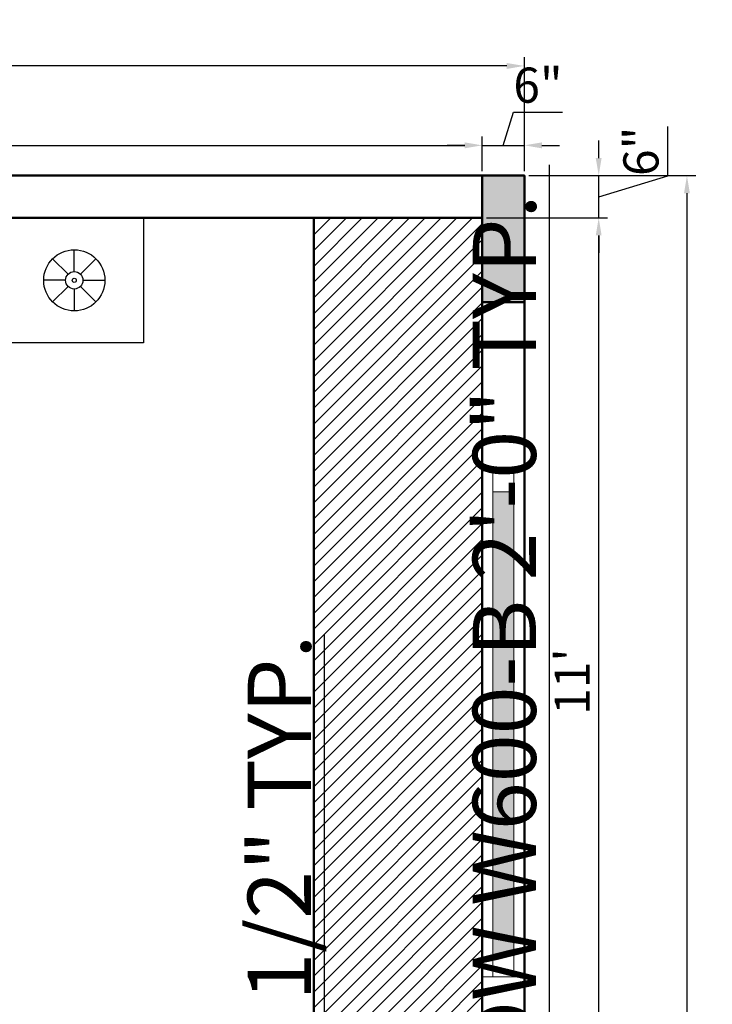
# Model space of a CAD drawing. Units: inches. Extents: x 3064 to 19385, y 846 to 15425.
# Tile 79 of 108: x 6739 to 6838, y 1870 to 2010. Entities that reach past the tile are written whole.
import ezdxf

# ---------------------------------------------------------------- set-up
doc = ezdxf.new("R2010")
doc.units = ezdxf.units.IN
for name, color, linetype, lineweight in [('A-ANNO-DIMS', 2, 'Continuous', 18), ('A-COLS', 1, 'Continuous', 35), ('A-FLOR-FIXT', 9, 'Continuous', 18), ('A-FURN-PATT', 252, 'Continuous', 13), ('A-GLAZ', 4, 'Continuous', 18), ('A-WALL', 7, 'Continuous', 50)]:
    doc.layers.add(name, color=color, linetype=linetype, lineweight=lineweight)
doc.layers.add('BLOCK', color=6, linetype='Continuous')
doc.styles.get("Standard").update_dxf_attribs({"font": 'arial.ttf'})
doc.dimstyles.new('ISO-25', dxfattribs={"dimtxt": 9, "dimasz": 2.5, "dimexe": 1.25, "dimexo": 0.625, "dimtad": 1, "dimdec": 1, "dimlunit": 3, "dimtxsty": 'Standard', "dimcen": 2.5, "dimadec": 0, "dimazin": 0, "dimtfac": 1, "dimtdec": 1, "dimtmove": 0, "dimatfit": 3, "dimfxl": 1, "dimarcsym": 0})

# ---------------------------------------------------------------- blocks, each defined once
blk = doc.blocks.new('A$C52E67D0D')
at = {"layer": 'BLOCK'}
for p, q in [((2251.5, 1605.5), (2251.5, 1684.7)), ((2229.3, 1596.3), (2173.3, 1652.3)), ((2273.7, 1596.3), (2329.7, 1652.3)), ((2220.1, 1574.1), (2140.9, 1574.1)), ((2282.9, 1574.1), (2362.1, 1574.1)), ((2229.3, 1551.9), (2173.3, 1495.9)), ((2251.5, 1542.8), (2251.5, 1463.5)), ((2273.7, 1551.9), (2329.7, 1495.9))]:
    blk.add_line(p, q, dxfattribs=at)
blk.add_lwpolyline([(2001, 1348.6), (2001, 1799.6), (2502, 1799.6), (2502, 1348.6)], close=True, dxfattribs=at)
for radius in [110.6, 31.4, 7.46]:
    blk.add_circle((2251.5, 1574.1), radius, dxfattribs=at)
blk = doc.blocks.new('*D346')
at = {"layer": 'A-ANNO-DIMS', "color": 0, "lineweight": -2, "transparency": 16777216}
for p, q in [((6805.66, 1981.99), (6822.87, 1981.99)), ((6821.62, 1852.49), (6821.62, 1979.49)), ((6811.66, 1849.99), (6822.87, 1849.99))]:
    blk.add_line(p, q, dxfattribs=at)
at = {"layer": 'A-ANNO-DIMS', "color": 0, "transparency": 16777216}
for points in [[(6821.2, 1979.49), (6822.03, 1979.49), (6821.62, 1981.99)], [(6821.2, 1852.49), (6822.03, 1852.49), (6821.62, 1849.99)]]:
    blk.add_solid(points, dxfattribs=at)
at = {"layer": 'Defpoints', "color": 0, "transparency": 16777216}
for p in [(6805.03, 1981.99), (6821.62, 1981.99), (6811.03, 1849.99)]:
    blk.add_point(p, dxfattribs=at)
at = {"layer": 'A-ANNO-DIMS', "color": 0, "transparency": 16777216, "insert": (6818.48, 1915.99), "char_height": 5, "attachment_point": 5, "rotation": 90}
blk.add_mtext("11'", dxfattribs=at)
blk = doc.blocks.new('*D347')
at = {"layer": 'A-ANNO-DIMS', "color": 0, "lineweight": -2, "transparency": 16777216}
for p, q in [((6831.46, 1987.94), (6831.46, 1994.97)), ((6821.62, 1990.49), (6821.62, 1992.99)), ((6811.66, 1987.99), (6822.87, 1987.99)), ((6821.62, 1981.99), (6821.62, 1987.99)), ((6821.62, 1981.99), (6821.62, 1987.99)), ((6821.62, 1984.99), (6831.46, 1987.94)), ((6805.66, 1981.99), (6822.87, 1981.99)), ((6821.62, 1979.49), (6821.62, 1976.99))]:
    blk.add_line(p, q, dxfattribs=at)
at = {"layer": 'A-ANNO-DIMS', "color": 0, "transparency": 16777216}
for points in [[(6821.2, 1990.49), (6822.03, 1990.49), (6821.62, 1987.99)], [(6821.2, 1979.49), (6822.03, 1979.49), (6821.62, 1981.99)]]:
    blk.add_solid(points, dxfattribs=at)
at = {"layer": 'Defpoints', "color": 0, "transparency": 16777216}
for p in [(6811.03, 1987.99), (6821.62, 1987.99), (6805.03, 1981.99)]:
    blk.add_point(p, dxfattribs=at)
at = {"layer": 'A-ANNO-DIMS', "color": 0, "transparency": 16777216, "insert": (6828.28, 1991.45), "char_height": 5, "attachment_point": 5, "rotation": 90}
blk.add_mtext('6"', dxfattribs=at)
blk = doc.blocks.new('*D348')
at = {"layer": 'A-ANNO-DIMS', "color": 0, "lineweight": -2, "transparency": 16777216}
for p, q in [((6811.66, 1987.99), (6835.44, 1987.99)), ((6834.19, 1985.49), (6834.19, 1498.49)), ((6811.66, 1495.99), (6835.44, 1495.99))]:
    blk.add_line(p, q, dxfattribs=at)
at = {"layer": 'A-ANNO-DIMS', "color": 0, "transparency": 16777216}
for points in [[(6833.77, 1985.49), (6834.6, 1985.49), (6834.19, 1987.99)], [(6833.77, 1498.49), (6834.6, 1498.49), (6834.19, 1495.99)]]:
    blk.add_solid(points, dxfattribs=at)
at = {"layer": 'Defpoints', "color": 0, "transparency": 16777216}
for p in [(6811.03, 1987.99), (6811.03, 1495.99), (6834.19, 1495.99)]:
    blk.add_point(p, dxfattribs=at)
at = {"layer": 'A-ANNO-DIMS', "color": 0, "transparency": 16777216, "insert": (6831.05, 1741.99), "char_height": 5, "attachment_point": 5, "rotation": 90}
blk.add_mtext("41'", dxfattribs=at)
blk = doc.blocks.new('*D344')
at = {"layer": 'A-ANNO-DIMS', "color": 0, "lineweight": -2, "transparency": 16777216}
for p, q in [((6610.03, 1988.61), (6610.03, 1993.55)), ((6805.03, 1988.61), (6805.03, 1993.55)), ((6612.53, 1992.3), (6802.53, 1992.3))]:
    blk.add_line(p, q, dxfattribs=at)
at = {"layer": 'A-ANNO-DIMS', "color": 0, "transparency": 16777216}
for points in [[(6612.53, 1992.72), (6612.53, 1991.88), (6610.03, 1992.3)], [(6802.53, 1992.72), (6802.53, 1991.88), (6805.03, 1992.3)]]:
    blk.add_solid(points, dxfattribs=at)
at = {"layer": 'Defpoints', "color": 0, "transparency": 16777216}
for p in [(6805.03, 1992.3), (6610.03, 1987.99), (6805.03, 1987.99)]:
    blk.add_point(p, dxfattribs=at)
at = {"layer": 'A-ANNO-DIMS', "color": 0, "transparency": 16777216, "insert": (6707.53, 1995.48), "char_height": 5, "attachment_point": 5}
blk.add_mtext('16\'-3"', dxfattribs=at)
blk = doc.blocks.new('*D345')
at = {"layer": 'A-ANNO-DIMS', "color": 0, "lineweight": -2, "transparency": 16777216}
for p, q in [((6808.03, 1992.3), (6809.46, 1997.04)), ((6809.46, 1997.04), (6816.48, 1997.04)), ((6805.03, 1988.61), (6805.03, 1993.55)), ((6811.03, 1988.61), (6811.03, 1993.55)), ((6802.53, 1992.3), (6800.03, 1992.3)), ((6805.03, 1992.3), (6811.03, 1992.3)), ((6805.03, 1992.3), (6811.03, 1992.3)), ((6813.53, 1992.3), (6816.03, 1992.3))]:
    blk.add_line(p, q, dxfattribs=at)
at = {"layer": 'A-ANNO-DIMS', "color": 0, "transparency": 16777216}
for points in [[(6802.53, 1992.72), (6802.53, 1991.88), (6805.03, 1992.3)], [(6813.53, 1992.72), (6813.53, 1991.88), (6811.03, 1992.3)]]:
    blk.add_solid(points, dxfattribs=at)
at = {"layer": 'Defpoints', "color": 0, "transparency": 16777216}
for p in [(6811.03, 1992.3), (6805.03, 1987.99), (6811.03, 1987.99)]:
    blk.add_point(p, dxfattribs=at)
at = {"layer": 'A-ANNO-DIMS', "color": 0, "transparency": 16777216, "insert": (6812.97, 2000.22), "char_height": 5, "attachment_point": 5}
blk.add_mtext('6"', dxfattribs=at)
blk = doc.blocks.new('*D340')
at = {"layer": 'A-ANNO-DIMS', "color": 0, "lineweight": -2, "transparency": 16777216}
for p, q in [((6469.03, 1988.61), (6469.03, 2004.85)), ((6811.03, 1988.61), (6811.03, 2004.85)), ((6808.53, 2003.6), (6471.53, 2003.6))]:
    blk.add_line(p, q, dxfattribs=at)
at = {"layer": 'A-ANNO-DIMS', "color": 0, "transparency": 16777216}
for points in [[(6471.53, 2004.02), (6471.53, 2003.18), (6469.03, 2003.6)], [(6808.53, 2004.02), (6808.53, 2003.18), (6811.03, 2003.6)]]:
    blk.add_solid(points, dxfattribs=at)
at = {"layer": 'Defpoints', "color": 0, "transparency": 16777216}
for p in [(6469.03, 2003.6), (6469.03, 1987.99), (6811.03, 1987.99)]:
    blk.add_point(p, dxfattribs=at)
at = {"layer": 'A-ANNO-DIMS', "color": 0, "transparency": 16777216, "insert": (6640.03, 2006.78), "char_height": 5, "attachment_point": 5}
blk.add_mtext('28\'-6"', dxfattribs=at)
blk = doc.blocks.new('WIN-1900-A')
h = blk.add_hatch(color=256)
h.dxf.hatch_style = 1
h.paths.add_polyline_path([(1.5, 0), (4.5, 0), (4.5, 66), (1.5, 66)])
for p, q in [((0, 69), (6, 69)), ((1.5, 66), (1.5, 0)), ((4.5, 66), (4.5, 0))]:
    blk.add_line(p, q)
blk.add_lwpolyline([(4.5, 66), (1.5, 66), (1.5, 69), (4.5, 69)], close=True)
blk = doc.blocks.new('*D404')
at = {"layer": 'A-ANNO-DIMS', "color": 0, "lineweight": -2, "transparency": 16777216}
for p, q in [((6782.57, 1843.99), (6782.57, 1922.72)), ((6780.81, 1843.99), (6783.82, 1843.99)), ((6782.57, 1832.8), (6782.57, 1841.49)), ((6780.81, 1830.3), (6783.82, 1830.3))]:
    blk.add_line(p, q, dxfattribs=at)
at = {"layer": 'A-ANNO-DIMS', "color": 0, "transparency": 16777216}
for points in [[(6782.16, 1841.49), (6782.99, 1841.49), (6782.57, 1843.99)], [(6782.16, 1832.8), (6782.99, 1832.8), (6782.57, 1830.3)]]:
    blk.add_solid(points, dxfattribs=at)
at = {"layer": 'Defpoints', "color": 0, "transparency": 16777216}
for p in [(6780.18, 1843.99), (6782.57, 1843.99), (6780.18, 1830.3)]:
    blk.add_point(p, dxfattribs=at)
at = {"layer": 'A-ANNO-DIMS', "color": 0, "transparency": 16777216, "insert": (6777.29, 1884.61), "char_height": 9, "attachment_point": 5, "rotation": 90}
blk.add_mtext('1\'-1 1/2" TYP.', dxfattribs=at)
blk = doc.blocks.new('*D441')
at = {"layer": 'A-ANNO-DIMS', "color": 0, "lineweight": -2, "transparency": 16777216}
for p, q in [((6814.63, 1822.99), (6814.63, 1989.54)), ((6811.66, 1822.99), (6815.88, 1822.99)), ((6814.63, 1801.49), (6814.63, 1820.49)), ((6811.66, 1798.99), (6815.88, 1798.99))]:
    blk.add_line(p, q, dxfattribs=at)
at = {"layer": 'A-ANNO-DIMS', "color": 0, "transparency": 16777216}
for points in [[(6814.22, 1820.49), (6815.05, 1820.49), (6814.63, 1822.99)], [(6814.22, 1801.49), (6815.05, 1801.49), (6814.63, 1798.99)]]:
    blk.add_solid(points, dxfattribs=at)
at = {"layer": 'Defpoints', "color": 0, "transparency": 16777216}
for p in [(6811.03, 1822.99), (6814.63, 1822.99), (6811.03, 1798.99)]:
    blk.add_point(p, dxfattribs=at)
at = {"layer": 'A-ANNO-DIMS', "color": 0, "transparency": 16777216, "insert": (6809.35, 1907.51), "char_height": 9, "attachment_point": 5, "rotation": 90}
blk.add_mtext('WINDOW W600-B 2\'-0" TYP.', dxfattribs=at)

msp = doc.modelspace()

# ---------------------------------------------------------------- hatches: boundary and pattern name
at = {"layer": 'A-COLS'}
h = msp.add_hatch(color=256, dxfattribs=at)
h.dxf.hatch_style = 1
h.paths.add_polyline_path([(6805.03, 1969.99), (6811.03, 1969.99), (6811.03, 1987.99), (6805.03, 1987.99)])
at = {"layer": 'A-FURN-PATT'}
h = msp.add_hatch(dxfattribs=at)
h.set_pattern_fill('ANSI31', color=256, scale=0.5)
h.set_pattern_definition([(45, (2126.5405, 591.649), (-1.122532, 1.122532), [])])
h.paths.add_polyline_path([(6781.03, 1849.99), (6805.03, 1849.99), (6805.03, 1981.99), (6781.03, 1981.99)])

# ---------------------------------------------------------------- linework, layer by layer
at = {"layer": 'A-GLAZ'}
msp.add_line((6811.03, 1873.99), (6805.03, 1873.99), dxfattribs=at)
msp.add_lwpolyline([(6809.53, 1873.99), (6806.53, 1873.99), (6806.53, 1876.99), (6809.53, 1876.99)], close=True, dxfattribs=at)
at = {"layer": 'A-WALL'}
for p, q in [((6811.03, 1987.99), (6469.03, 1987.99)), ((6811.03, 1495.99), (6811.03, 1987.99)), ((6805.03, 1981.99), (6610.03, 1981.99)), ((6781.03, 1849.99), (6781.03, 1981.99)), ((6805.03, 1849.99), (6805.03, 1981.99))]:
    msp.add_line(p, q, dxfattribs=at)
msp.add_lwpolyline([(6811.03, 1969.99), (6811.03, 1987.99), (6805.03, 1987.99), (6805.03, 1969.99)], close=True, dxfattribs=at)

# ---------------------------------------------------------------- block references
at = {"layer": 'A-FLOR-FIXT', "xscale": 0.039370099999992, "yscale": 0.039370099999992, "zscale": 0.039370099999992}
msp.add_blockref('A$C52E67D0D', (6658.28, 1911.12), dxfattribs=at)
at = {"layer": 'A-GLAZ'}
msp.add_blockref('WIN-1900-A', (6805.03, 1876.99), dxfattribs=at)

# ---------------------------------------------------------------- dimensions: what is measured, and where the dimension line sits
at = {"layer": 'A-ANNO-DIMS'}
for base, p1, p2, override, picture, middle in [((6469.03, 2003.6), (6811.03, 1987.99), (6469.03, 1987.99), {"dimtxt": 5, "dimclrd": 0, "dimclre": 0, "dimclrt": 0}, '*D340', (6640.03, 2006.78)), ((6811.03, 1992.3), (6805.03, 1987.99), (6811.03, 1987.99), {"dimtxt": 5, "dimclrd": 0, "dimclre": 0, "dimclrt": 0, "dimtmove": 1}, '*D345', (6810.08, 2000.22)), ((6805.03, 1992.3), (6610.03, 1987.99), (6805.03, 1987.99), {"dimtxt": 5, "dimclrd": 0, "dimclre": 0, "dimclrt": 0, "dimtmove": 1}, '*D344', (6707.53, 1995.48))]:
    dim = msp.add_linear_dim(base=base, p1=p1, p2=p2, dimstyle='ISO-25', override=override, dxfattribs=at)
    dim.commit()
    dim.dimension.update_dxf_attribs({"geometry": picture, "text_midpoint": middle})
for base, p1, p2, override, picture, middle in [((6821.62, 1987.99), (6805.03, 1981.99), (6811.03, 1987.99), {"dimtxt": 5, "dimclrd": 0, "dimclre": 0, "dimclrt": 0, "dimtmove": 1}, '*D347', (6828.28, 1988.57)), ((6834.19, 1495.99), (6811.03, 1987.99), (6811.03, 1495.99), {"dimtxt": 5, "dimclrd": 0, "dimclre": 0, "dimclrt": 0}, '*D348', (6831.05, 1741.99)), ((6821.62, 1981.99), (6811.03, 1849.99), (6805.03, 1981.99), {"dimtxt": 5, "dimclrd": 0, "dimclre": 0, "dimclrt": 0, "dimtmove": 1}, '*D346', (6818.48, 1915.99))]:
    dim = msp.add_linear_dim(base=base, p1=p1, p2=p2, angle=90, dimstyle='ISO-25', override=override, dxfattribs=at)
    dim.commit()
    dim.dimension.update_dxf_attribs({"geometry": picture, "text_midpoint": middle})
for base, p1, p2, text, picture, middle in [((6814.63, 1822.99), (6811.03, 1798.99), (6811.03, 1822.99), 'WINDOW W600-B <> TYP.', '*D441', (6809.35, 1907.51)), ((6782.57, 1843.99), (6780.18, 1830.3), (6780.18, 1843.99), '<> TYP.', '*D404', (6777.29, 1884.61))]:
    dim = msp.add_linear_dim(base=base, p1=p1, p2=p2, angle=90, text=text, dimstyle='ISO-25', override={"dimdec": 1, "dimrnd": 0, "dimzin": 1, "dimlunit": 4, "dimfrac": 2}, dxfattribs=at)
    dim.commit()
    dim.dimension.update_dxf_attribs({"geometry": picture, "text_midpoint": middle})

doc.saveas('drawing.dxf')
